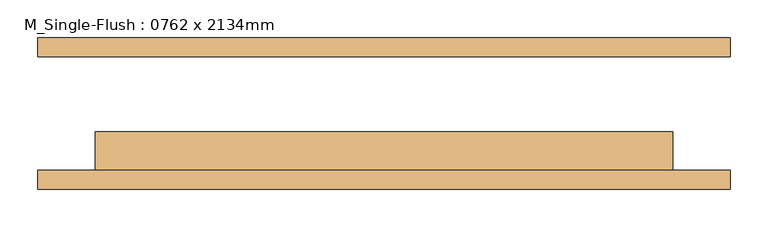
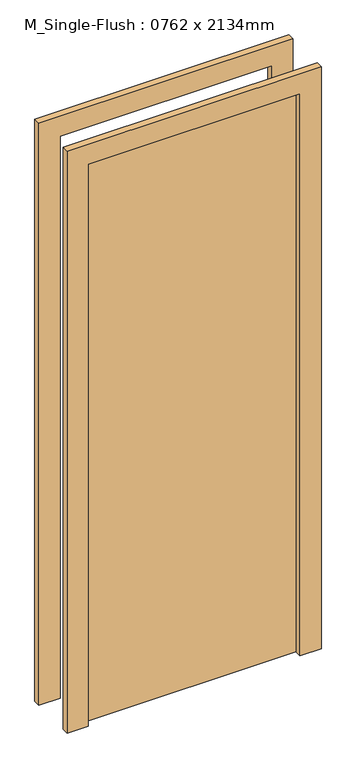
"""IFC4 building model written with IfcOpenShell, lengths in millimetres: door geometry, M_Single-Flush : 0762 x 2134mm."""

from ifc_helpers import new_model, si_unit, frame, origin, origin_with_axes, place, context, project, spatial, polyline, outline, extrude, source, transform, mapped, element, save


def m_single_flush_0762_x_2134mm_8c18b9de(model_context):
    return source(origin(), model_context, "Body", "SweptSolid", [
        extrude(outline(polyline([(2210.0, -457.0), (0.0, -457.0), (0.0, -381.0), (2134.0, -381.0), (2134.0, 381.0), (0.0, 381.0), (0.0, 457.0), (2210.0, 457.0), (2210.0, -457.0)])), frame((0.0, -100.0, 0.0), z_axis=(0.0, 1.0, 0.0), x_axis=(0.0, 0.0, 1.0)), (0.0, 0.0, 1.0), 25.0),
        extrude(outline(polyline([(2210.0, 457.0), (2210.0, -457.0), (0.0, -457.0), (0.0, -381.0), (2134.0, -381.0), (2134.0, 381.0), (0.0, 381.0), (0.0, 457.0), (2210.0, 457.0)])), frame((0.0, 75.0, 0.0), z_axis=(0.0, 1.0, 0.0), x_axis=(0.0, 0.0, 1.0)), (0.0, 0.0, 1.0), 25.0),
        extrude(outline(polyline([(381.0, -24.0), (381.0, -75.0), (-381.0, -75.0), (-381.0, -24.0), (381.0, -24.0)])), origin_with_axes(), (0.0, 0.0, 1.0), 2134.0),
    ])


if __name__ == "__main__":
    model = new_model("IFC4")
    model_context = context("Model", 3, world=origin())
    ifc_project = project(units=[si_unit("LENGTHUNIT", "METRE", prefix="MILLI")], contexts=[model_context])
    site = spatial("IfcSite", under=ifc_project)
    building = spatial("IfcBuilding", under=site)
    placement = place(None, origin())
    m_single_flush_0762_x_2134mm_shape = m_single_flush_0762_x_2134mm_8c18b9de(model_context)
    element("IfcDoor", 1, ObjectType="M_Single-Flush : 0762 x 2134mm", at=placement, inside=building, context=model_context, shape_type="MappedRepresentation", body=[
        mapped(m_single_flush_0762_x_2134mm_shape, transform((0.0, 0.0, 0.0), x_axis=(1.0, 0.0, 0.0), y_axis=(0.0, 1.0, 0.0), z_axis=(0.0, 0.0, 1.0))),
    ])
    save(model, "model.ifc")

# Revit data of these elements
# Type "M_Single-Flush : 0762 x 2134mm"
#   Type Mark = "26"
#   Construction Type Id = "MDOOR"
#   Analytic Construction = "Metal"
#   Thickness = 0.051 m
#   Thermal Resistance (R) = 0.270117 (m²·K)/W
#   Heat Transfer Coefficient (U) = 3.7021 W/(m²·K)
#   Height = 2.134 m
#   Trim Projection Ext = 0.025 m
#   Trim Projection Int = 0.025 m
#   Trim Width = 0.076 m
#   Width = 0.762 m
#   Define Thermal Properties by = 1
#   Define Thermal Properties by = 1
#   Door Material = Door - Panel
#   Frame Material = Door - Frame
#   Visual Light Transmittance = 0
#   Solar Heat Gain Coefficient = 0
#   Function = (empty or 0)
#   Wall Closure = (empty or 0)
# Element 1 (IfcDoor, "M_Single-Flush : 0762 x 2134mm")
#   Materials on its faces: "Door - Frame", "Door - Panel"
# Materials
#   "Door - Panel": class "Wood", colour RGB 210 159 95, transparency 0, Cost = 0
#   "Door - Frame": colour RGB 118 70 51, transparency 0, Cost = 0
